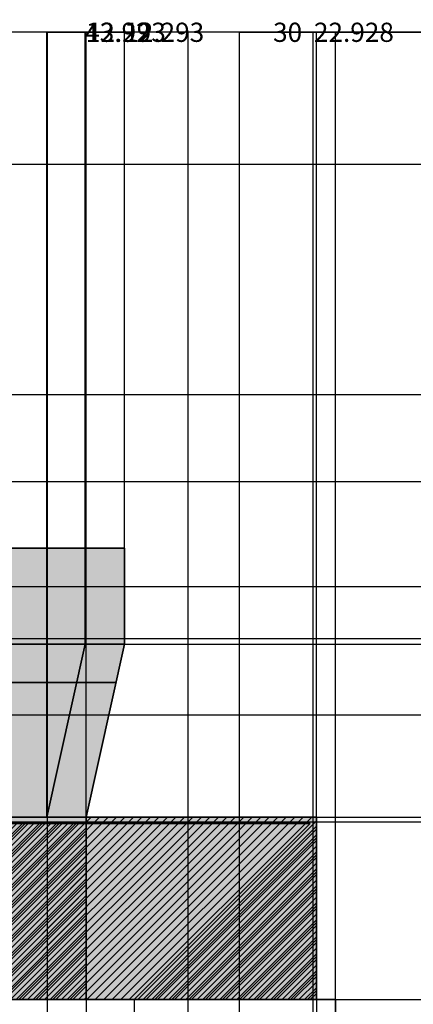
# Model space of a CAD drawing. Units: inches. Extents: x 148 to 1080, y 89 to 707.
# Tile 11 of 12: x 674 to 797, y 399 to 707. Entities that reach past the tile are written whole.
import ezdxf

# ---------------------------------------------------------------- set-up
doc = ezdxf.new("R2010")
doc.units = ezdxf.units.IN
doc.header["$MEASUREMENT"] = 0
for name, color, linetype, lineweight in [('A-ANNO-DIMS', 2, 'Continuous', 18), ('A-ELEV', 7, 'Continuous', 35), ('A-ELEV-PATT', 8, 'Continuous', 13)]:
    doc.layers.add(name, color=color, linetype=linetype, lineweight=lineweight)
doc.styles.get("Standard").update_dxf_attribs({"font": 'arial.ttf'})
doc.dimstyles.get("Standard").update_dxf_attribs({"dimtxt": 6, "dimasz": 0.18, "dimexe": 0.18, "dimexo": 0.0625, "dimgap": 0.09, "dimtad": 0, "dimtih": 1, "dimtoh": 1, "dimdec": 0, "dimzin": 0, "dimdsep": 46, "dimlunit": 3, "dimtxsty": 'Standard', "dimcen": 0.09, "dimadec": 0, "dimazin": 0, "dimtfac": 1, "dimtdec": 0, "dimtofl": 0, "dimtmove": 0, "dimatfit": 3, "dimfxl": 1, "dimtolj": 1, "dimtzin": 0, "dimarcsym": 0})

# ---------------------------------------------------------------- blocks, each defined once
blk = doc.blocks.new('*D1')
at = {"layer": 'A-ANNO-DIMS', "color": 0, "lineweight": -2, "transparency": 16777216}
for p, q in [((215.02, 662.01), (215.02, 703.28)), ((215.2, 703.1), (604.32, 703.1)), ((1006.77, 703.1), (617.65, 703.1)), ((1006.95, 338.01), (1006.95, 703.28))]:
    blk.add_line(p, q, dxfattribs=at)
at = {"layer": 'A-ANNO-DIMS', "color": 0, "transparency": 16777216}
for points in [[(215.2, 703.13), (215.2, 703.07), (215.02, 703.1)], [(1006.77, 703.13), (1006.77, 703.07), (1006.95, 703.1)]]:
    blk.add_solid(points, dxfattribs=at)
at = {"layer": 'Defpoints', "color": 0, "transparency": 16777216}
for p in [(1006.95, 703.1), (215.02, 661.95), (1006.95, 337.95)]:
    blk.add_point(p, dxfattribs=at)
at = {"layer": 'A-ANNO-DIMS', "color": 0, "transparency": 16777216, "insert": (610.98, 703.1), "char_height": 6, "attachment_point": 5}
blk.add_mtext('\\A1;792', dxfattribs=at)
blk = doc.blocks.new('*D14')
at = {"layer": 'A-ANNO-DIMS', "color": 0, "lineweight": -2, "transparency": 16777216}
for p, q in [((611.02, 542.01), (611.02, 703.28)), ((611.2, 703.1), (654.63, 703.1)), ((706.84, 703.1), (663.41, 703.1)), ((707.02, 542.01), (707.02, 703.28))]:
    blk.add_line(p, q, dxfattribs=at)
at = {"layer": 'A-ANNO-DIMS', "color": 0, "transparency": 16777216}
for points in [[(611.2, 703.13), (611.2, 703.07), (611.02, 703.1)], [(706.84, 703.13), (706.84, 703.07), (707.02, 703.1)]]:
    blk.add_solid(points, dxfattribs=at)
at = {"layer": 'Defpoints', "color": 0, "transparency": 16777216}
for p in [(707.02, 703.1), (611.02, 541.95), (707.02, 541.95)]:
    blk.add_point(p, dxfattribs=at)
at = {"layer": 'A-ANNO-DIMS', "color": 0, "transparency": 16777216, "insert": (659.02, 703.1), "char_height": 6, "attachment_point": 5}
blk.add_mtext('\\A1;96', dxfattribs=at)
blk = doc.blocks.new('*D16')
at = {"layer": 'A-ANNO-DIMS', "color": 0, "lineweight": -2, "transparency": 16777216}
for p, q in [((527.02, 458.01), (527.02, 703.28)), ((527.2, 703.1), (640.26, 703.1)), ((766.84, 703.1), (653.78, 703.1)), ((767.02, 458.01), (767.02, 703.28))]:
    blk.add_line(p, q, dxfattribs=at)
at = {"layer": 'A-ANNO-DIMS', "color": 0, "transparency": 16777216}
for points in [[(527.2, 703.13), (527.2, 703.07), (527.02, 703.1)], [(766.84, 703.13), (766.84, 703.07), (767.02, 703.1)]]:
    blk.add_solid(points, dxfattribs=at)
at = {"layer": 'Defpoints', "color": 0, "transparency": 16777216}
for p in [(767.02, 703.1), (527.02, 457.95), (767.02, 457.95)]:
    blk.add_point(p, dxfattribs=at)
at = {"layer": 'A-ANNO-DIMS', "color": 0, "transparency": 16777216, "insert": (647.02, 703.1), "char_height": 6, "attachment_point": 5}
blk.add_mtext('\\A1;240', dxfattribs=at)
blk = doc.blocks.new('*D17')
at = {"layer": 'A-ANNO-DIMS', "color": 0, "lineweight": -2, "transparency": 16777216}
for p, q in [((743.02, 338.01), (743.02, 703.28)), ((743.2, 703.1), (753.64, 703.1)), ((772.84, 703.1), (762.39, 703.1)), ((773.02, 368.01), (773.02, 703.28))]:
    blk.add_line(p, q, dxfattribs=at)
at = {"layer": 'A-ANNO-DIMS', "color": 0, "transparency": 16777216}
for points in [[(743.2, 703.13), (743.2, 703.07), (743.02, 703.1)], [(772.84, 703.13), (772.84, 703.07), (773.02, 703.1)]]:
    blk.add_solid(points, dxfattribs=at)
at = {"layer": 'Defpoints', "color": 0, "transparency": 16777216}
for p in [(773.02, 703.1), (773.02, 367.95), (743.02, 337.95)]:
    blk.add_point(p, dxfattribs=at)
at = {"layer": 'A-ANNO-DIMS', "color": 0, "transparency": 16777216, "insert": (758.02, 703.1), "char_height": 6, "attachment_point": 5}
blk.add_mtext('\\A1;30', dxfattribs=at)
blk = doc.blocks.new('*D18')
at = {"layer": 'A-ANNO-DIMS', "color": 0, "lineweight": -2, "transparency": 16777216}
for p, q in [((635.08, 661.95), (1064.5, 661.95)), ((1064.32, 661.77), (1064.32, 401.1)), ((1064.32, 134.13), (1064.32, 394.79)), ((1007.01, 133.95), (1064.5, 133.95))]:
    blk.add_line(p, q, dxfattribs=at)
at = {"layer": 'A-ANNO-DIMS', "color": 0, "transparency": 16777216}
for points in [[(1064.29, 661.77), (1064.35, 661.77), (1064.32, 661.95)], [(1064.29, 134.13), (1064.35, 134.13), (1064.32, 133.95)]]:
    blk.add_solid(points, dxfattribs=at)
at = {"layer": 'Defpoints', "color": 0, "transparency": 16777216}
for p in [(635.02, 661.95), (1064.32, 661.95), (1006.95, 133.95)]:
    blk.add_point(p, dxfattribs=at)
at = {"layer": 'A-ANNO-DIMS', "color": 0, "transparency": 16777216, "insert": (1064.32, 397.95), "char_height": 6, "attachment_point": 5}
blk.add_mtext('\\A1;528', dxfattribs=at)
blk = doc.blocks.new('*D35')
at = {"layer": 'A-ANNO-DIMS', "color": 0, "lineweight": -2, "transparency": 16777216}
for p, q in [((743.02, 272.01), (743.02, 703.28)), ((743.2, 703.1), (765.77, 703.1)), ((765.95, 241.16), (765.95, 703.28)), ((765.95, 703.1), (766.13, 703.1))]:
    blk.add_line(p, q, dxfattribs=at)
at = {"layer": 'A-ANNO-DIMS', "color": 0, "transparency": 16777216}
for points in [[(743.2, 703.13), (743.2, 703.07), (743.02, 703.1)], [(765.77, 703.13), (765.77, 703.07), (765.95, 703.1)]]:
    blk.add_solid(points, dxfattribs=at)
at = {"layer": 'Defpoints', "color": 0, "transparency": 16777216}
for p in [(765.95, 703.1), (743.02, 271.95), (765.95, 241.1)]:
    blk.add_point(p, dxfattribs=at)
at = {"layer": 'A-ANNO-DIMS', "color": 0, "transparency": 16777216, "insert": (778.73, 703.1), "char_height": 6, "attachment_point": 5}
blk.add_mtext('\\A1;22.928', dxfattribs=at)
blk = doc.blocks.new('*D36')
at = {"layer": 'A-ANNO-DIMS', "color": 0, "lineweight": -2, "transparency": 16777216}
for p, q in [((765.95, 241.16), (765.95, 703.28)), ((766.13, 703.1), (844.01, 703.1)), ((934.77, 703.1), (856.89, 703.1)), ((934.95, 272.01), (934.95, 703.28))]:
    blk.add_line(p, q, dxfattribs=at)
at = {"layer": 'A-ANNO-DIMS', "color": 0, "transparency": 16777216}
for points in [[(766.13, 703.13), (766.13, 703.07), (765.95, 703.1)], [(934.77, 703.13), (934.77, 703.07), (934.95, 703.1)]]:
    blk.add_solid(points, dxfattribs=at)
at = {"layer": 'Defpoints', "color": 0, "transparency": 16777216}
for p in [(934.95, 703.1), (934.95, 271.95), (765.95, 241.1)]:
    blk.add_point(p, dxfattribs=at)
at = {"layer": 'A-ANNO-DIMS', "color": 0, "transparency": 16777216, "insert": (850.45, 703.1), "char_height": 6, "attachment_point": 5}
blk.add_mtext('\\A1;169', dxfattribs=at)
blk = doc.blocks.new('*D37')
at = {"layer": 'A-ANNO-DIMS', "color": 0, "lineweight": -2, "transparency": 16777216}
for p, q in [((765.95, 241.16), (765.95, 703.28)), ((766.13, 703.1), (836.75, 703.1)), ((927.28, 703.1), (856.66, 703.1)), ((927.46, 240.26), (927.46, 703.28))]:
    blk.add_line(p, q, dxfattribs=at)
at = {"layer": 'A-ANNO-DIMS', "color": 0, "transparency": 16777216}
for points in [[(766.13, 703.13), (766.13, 703.07), (765.95, 703.1)], [(927.28, 703.13), (927.28, 703.07), (927.46, 703.1)]]:
    blk.add_solid(points, dxfattribs=at)
at = {"layer": 'Defpoints', "color": 0, "transparency": 16777216}
for p in [(927.46, 703.1), (765.95, 241.1), (927.46, 240.2)]:
    blk.add_point(p, dxfattribs=at)
at = {"layer": 'A-ANNO-DIMS', "color": 0, "transparency": 16777216, "insert": (846.7, 703.1), "char_height": 6, "attachment_point": 5}
blk.add_mtext('\\A1;161.5', dxfattribs=at)
blk = doc.blocks.new('*D47')
at = {"layer": 'A-ANNO-DIMS', "color": 0, "lineweight": -2, "transparency": 16777216}
for p, q in [((628.17, 353.26), (628.17, 703.28)), ((628.35, 703.1), (645.36, 703.1)), ((682.84, 703.1), (665.83, 703.1)), ((683.02, 338.01), (683.02, 703.28))]:
    blk.add_line(p, q, dxfattribs=at)
at = {"layer": 'A-ANNO-DIMS', "color": 0, "transparency": 16777216}
for points in [[(628.35, 703.13), (628.35, 703.07), (628.17, 703.1)], [(682.84, 703.13), (682.84, 703.07), (683.02, 703.1)]]:
    blk.add_solid(points, dxfattribs=at)
at = {"layer": 'Defpoints', "color": 0, "transparency": 16777216}
for p in [(683.02, 703.1), (628.17, 353.2), (683.02, 337.95)]:
    blk.add_point(p, dxfattribs=at)
at = {"layer": 'A-ANNO-DIMS', "color": 0, "transparency": 16777216, "insert": (655.6, 703.1), "char_height": 6, "attachment_point": 5}
blk.add_mtext('\\A1;54.85', dxfattribs=at)
blk = doc.blocks.new('*D48')
at = {"layer": 'A-ANNO-DIMS', "color": 0, "lineweight": -2, "transparency": 16777216}
for p, q in [((683.02, 338.01), (683.02, 703.28)), ((683.2, 703.1), (694.68, 703.1)), ((726.76, 703.1), (715.28, 703.1)), ((726.94, 354.92), (726.94, 703.28))]:
    blk.add_line(p, q, dxfattribs=at)
at = {"layer": 'A-ANNO-DIMS', "color": 0, "transparency": 16777216}
for points in [[(683.2, 703.13), (683.2, 703.07), (683.02, 703.1)], [(726.76, 703.13), (726.76, 703.07), (726.94, 703.1)]]:
    blk.add_solid(points, dxfattribs=at)
at = {"layer": 'Defpoints', "color": 0, "transparency": 16777216}
for p in [(726.94, 703.1), (726.94, 354.86), (683.02, 337.95)]:
    blk.add_point(p, dxfattribs=at)
at = {"layer": 'A-ANNO-DIMS', "color": 0, "transparency": 16777216, "insert": (704.98, 703.1), "char_height": 6, "attachment_point": 5}
blk.add_mtext('\\A1;43.92', dxfattribs=at)
blk = doc.blocks.new('*D51')
at = {"layer": 'A-ANNO-DIMS', "color": 0, "lineweight": -2, "transparency": 16777216}
for p, q in [((707.08, 511.95), (1064.5, 511.95)), ((1064.32, 511.77), (1064.32, 488.1)), ((1064.32, 458.13), (1064.32, 481.79)), ((695.08, 457.95), (1064.5, 457.95))]:
    blk.add_line(p, q, dxfattribs=at)
at = {"layer": 'A-ANNO-DIMS', "color": 0, "transparency": 16777216}
for points in [[(1064.29, 511.77), (1064.35, 511.77), (1064.32, 511.95)], [(1064.29, 458.13), (1064.35, 458.13), (1064.32, 457.95)]]:
    blk.add_solid(points, dxfattribs=at)
at = {"layer": 'Defpoints', "color": 0, "transparency": 16777216}
for p in [(707.02, 511.95), (695.02, 457.95), (1064.32, 457.95)]:
    blk.add_point(p, dxfattribs=at)
at = {"layer": 'A-ANNO-DIMS', "color": 0, "transparency": 16777216, "insert": (1064.32, 484.95), "char_height": 6, "attachment_point": 5}
blk.add_mtext('\\A1;54.00', dxfattribs=at)
blk = doc.blocks.new('*D53')
at = {"layer": 'A-ANNO-DIMS', "color": 0, "lineweight": -2, "transparency": 16777216}
for p, q in [((694.73, 512.01), (694.73, 703.28)), ((694.91, 703.1), (706.84, 703.1)), ((707.02, 512.01), (707.02, 703.28)), ((707.02, 703.1), (707.2, 703.1))]:
    blk.add_line(p, q, dxfattribs=at)
at = {"layer": 'A-ANNO-DIMS', "color": 0, "transparency": 16777216}
for points in [[(694.91, 703.13), (694.91, 703.07), (694.73, 703.1)], [(706.84, 703.13), (706.84, 703.07), (707.02, 703.1)]]:
    blk.add_solid(points, dxfattribs=at)
at = {"layer": 'Defpoints', "color": 0, "transparency": 16777216}
for p in [(707.02, 703.1), (694.73, 511.95), (707.02, 511.95)]:
    blk.add_point(p, dxfattribs=at)
at = {"layer": 'A-ANNO-DIMS', "color": 0, "transparency": 16777216, "insert": (719.46, 703.1), "char_height": 6, "attachment_point": 5}
blk.add_mtext('\\A1;12.293', dxfattribs=at)
blk = doc.blocks.new('*D54')
at = {"layer": 'A-ANNO-DIMS', "color": 0, "lineweight": -2, "transparency": 16777216}
for p, q in [((682.73, 458.01), (682.73, 703.28)), ((682.91, 703.1), (694.84, 703.1)), ((695.02, 458.01), (695.02, 703.28)), ((695.02, 703.1), (695.2, 703.1))]:
    blk.add_line(p, q, dxfattribs=at)
at = {"layer": 'A-ANNO-DIMS', "color": 0, "transparency": 16777216}
for points in [[(682.91, 703.13), (682.91, 703.07), (682.73, 703.1)], [(694.84, 703.13), (694.84, 703.07), (695.02, 703.1)]]:
    blk.add_solid(points, dxfattribs=at)
at = {"layer": 'Defpoints', "color": 0, "transparency": 16777216}
for p in [(695.02, 703.1), (682.73, 457.95), (695.02, 457.95)]:
    blk.add_point(p, dxfattribs=at)
at = {"layer": 'A-ANNO-DIMS', "color": 0, "transparency": 16777216, "insert": (707.46, 703.1), "char_height": 6, "attachment_point": 5}
blk.add_mtext('\\A1;12.293', dxfattribs=at)
blk = doc.blocks.new('*D58')
at = {"layer": 'A-ANNO-DIMS', "color": 0, "lineweight": -2, "transparency": 16777216}
for p, q in [((611.02, 400.88), (611.02, 92.62)), ((695.02, 400.88), (695.02, 92.62)), ((611.2, 92.8), (642.81, 92.8)), ((694.84, 92.8), (663.23, 92.8))]:
    blk.add_line(p, q, dxfattribs=at)
at = {"layer": 'A-ANNO-DIMS', "color": 0, "transparency": 16777216}
for points in [[(611.2, 92.83), (611.2, 92.77), (611.02, 92.8)], [(694.84, 92.83), (694.84, 92.77), (695.02, 92.8)]]:
    blk.add_solid(points, dxfattribs=at)
at = {"layer": 'Defpoints', "color": 0, "transparency": 16777216}
for p in [(611.02, 400.95), (695.02, 400.95), (695.02, 92.8)]:
    blk.add_point(p, dxfattribs=at)
at = {"layer": 'A-ANNO-DIMS', "color": 0, "transparency": 16777216, "insert": (653.02, 92.8), "char_height": 6, "attachment_point": 5}
blk.add_mtext('\\A1;84.00', dxfattribs=at)
blk = doc.blocks.new('*D59')
at = {"layer": 'A-ANNO-DIMS', "color": 0, "lineweight": -2, "transparency": 16777216}
for p, q in [((695.02, 400.88), (695.02, 92.62)), ((767.02, 400.88), (767.02, 92.62)), ((695.2, 92.8), (720.84, 92.8)), ((766.84, 92.8), (741.2, 92.8))]:
    blk.add_line(p, q, dxfattribs=at)
at = {"layer": 'A-ANNO-DIMS', "color": 0, "transparency": 16777216}
for points in [[(695.2, 92.83), (695.2, 92.77), (695.02, 92.8)], [(766.84, 92.83), (766.84, 92.77), (767.02, 92.8)]]:
    blk.add_solid(points, dxfattribs=at)
at = {"layer": 'Defpoints', "color": 0, "transparency": 16777216}
for p in [(695.02, 400.95), (767.02, 400.95), (767.02, 92.8)]:
    blk.add_point(p, dxfattribs=at)
at = {"layer": 'A-ANNO-DIMS', "color": 0, "transparency": 16777216, "insert": (731.02, 92.8), "char_height": 6, "attachment_point": 5}
blk.add_mtext('\\A1;72.00', dxfattribs=at)
blk = doc.blocks.new('*D60')
at = {"layer": 'A-ANNO-DIMS', "color": 0, "lineweight": -2, "transparency": 16777216}
for p, q in [((695.02, 400.88), (695.02, 92.62)), ((710.1, 400.88), (710.1, 92.62)), ((695.2, 92.8), (709.92, 92.8)), ((710.1, 92.8), (710.28, 92.8))]:
    blk.add_line(p, q, dxfattribs=at)
at = {"layer": 'A-ANNO-DIMS', "color": 0, "transparency": 16777216}
for points in [[(695.2, 92.83), (695.2, 92.77), (695.02, 92.8)], [(709.92, 92.83), (709.92, 92.77), (710.1, 92.8)]]:
    blk.add_solid(points, dxfattribs=at)
at = {"layer": 'Defpoints', "color": 0, "transparency": 16777216}
for p in [(695.02, 400.95), (710.1, 400.95), (710.1, 92.8)]:
    blk.add_point(p, dxfattribs=at)
at = {"layer": 'A-ANNO-DIMS', "color": 0, "transparency": 16777216, "insert": (720.22, 92.8), "char_height": 6, "attachment_point": 5}
blk.add_mtext('\\A1;15.08', dxfattribs=at)
blk = doc.blocks.new('*D90')
at = {"layer": 'A-ANNO-DIMS', "color": 0, "lineweight": -2, "transparency": 16777216}
for p, q in [((527.08, 489.89), (1064.5, 489.89)), ((1064.32, 489.71), (1064.32, 448.57)), ((1064.32, 401.13), (1064.32, 442.27)), ((527.08, 400.95), (1064.5, 400.95))]:
    blk.add_line(p, q, dxfattribs=at)
at = {"layer": 'A-ANNO-DIMS', "color": 0, "transparency": 16777216}
for points in [[(1064.29, 489.71), (1064.35, 489.71), (1064.32, 489.89)], [(1064.29, 401.13), (1064.35, 401.13), (1064.32, 400.95)]]:
    blk.add_solid(points, dxfattribs=at)
at = {"layer": 'Defpoints', "color": 0, "transparency": 16777216}
for p in [(527.02, 489.89), (527.02, 400.95), (1064.32, 400.95)]:
    blk.add_point(p, dxfattribs=at)
at = {"layer": 'A-ANNO-DIMS', "color": 0, "transparency": 16777216, "insert": (1064.32, 445.42), "char_height": 6, "attachment_point": 5}
blk.add_mtext('\\A1;88.94', dxfattribs=at)
blk = doc.blocks.new('*D91')
at = {"layer": 'A-ANNO-DIMS', "color": 0, "lineweight": -2, "transparency": 16777216}
for p, q in [((479.08, 513.77), (1064.5, 513.77)), ((1064.32, 513.59), (1064.32, 460.51)), ((1064.32, 401.13), (1064.32, 454.21)), ((479.08, 400.95), (1064.5, 400.95))]:
    blk.add_line(p, q, dxfattribs=at)
at = {"layer": 'A-ANNO-DIMS', "color": 0, "transparency": 16777216}
for points in [[(1064.29, 513.59), (1064.35, 513.59), (1064.32, 513.77)], [(1064.29, 401.13), (1064.35, 401.13), (1064.32, 400.95)]]:
    blk.add_solid(points, dxfattribs=at)
at = {"layer": 'Defpoints', "color": 0, "transparency": 16777216}
for p in [(479.02, 513.77), (479.02, 400.95), (1064.32, 400.95)]:
    blk.add_point(p, dxfattribs=at)
at = {"layer": 'A-ANNO-DIMS', "color": 0, "transparency": 16777216, "insert": (1064.32, 457.36), "char_height": 6, "attachment_point": 5}
blk.add_mtext('\\A1;112.82', dxfattribs=at)
blk = doc.blocks.new('*D92')
at = {"layer": 'A-ANNO-DIMS', "color": 0, "lineweight": -2, "transparency": 16777216}
for p, q in [((389.08, 456.43), (1064.5, 456.43)), ((1064.32, 456.25), (1064.32, 431.84)), ((1064.32, 401.13), (1064.32, 425.53)), ((389.08, 400.95), (1064.5, 400.95))]:
    blk.add_line(p, q, dxfattribs=at)
at = {"layer": 'A-ANNO-DIMS', "color": 0, "transparency": 16777216}
for points in [[(1064.29, 456.25), (1064.35, 456.25), (1064.32, 456.43)], [(1064.29, 401.13), (1064.35, 401.13), (1064.32, 400.95)]]:
    blk.add_solid(points, dxfattribs=at)
at = {"layer": 'Defpoints', "color": 0, "transparency": 16777216}
for p in [(389.02, 456.43), (1064.32, 456.43), (389.02, 400.95)]:
    blk.add_point(p, dxfattribs=at)
at = {"layer": 'A-ANNO-DIMS', "color": 0, "transparency": 16777216, "insert": (1064.32, 428.69), "char_height": 6, "attachment_point": 5}
blk.add_mtext('\\A1;55.48', dxfattribs=at)
blk = doc.blocks.new('*D93')
at = {"layer": 'A-ANNO-DIMS', "color": 0, "lineweight": -2, "transparency": 16777216}
for p, q in [((389.08, 529.95), (1064.5, 529.95)), ((1064.32, 529.77), (1064.32, 496.34)), ((1064.32, 456.61), (1064.32, 490.03)), ((389.08, 456.43), (1064.5, 456.43))]:
    blk.add_line(p, q, dxfattribs=at)
at = {"layer": 'A-ANNO-DIMS', "color": 0, "transparency": 16777216}
for points in [[(1064.29, 529.77), (1064.35, 529.77), (1064.32, 529.95)], [(1064.29, 456.61), (1064.35, 456.61), (1064.32, 456.43)]]:
    blk.add_solid(points, dxfattribs=at)
at = {"layer": 'Defpoints', "color": 0, "transparency": 16777216}
for p in [(389.02, 529.95), (1064.32, 529.95), (389.02, 456.43)]:
    blk.add_point(p, dxfattribs=at)
at = {"layer": 'A-ANNO-DIMS', "color": 0, "transparency": 16777216, "insert": (1064.32, 493.19), "char_height": 6, "attachment_point": 5}
blk.add_mtext('\\A1;73.52', dxfattribs=at)
blk = doc.blocks.new('*D94')
at = {"layer": 'A-ANNO-DIMS', "color": 0, "lineweight": -2, "transparency": 16777216}
for p, q in [((389.08, 562.74), (1064.5, 562.74)), ((1064.32, 562.56), (1064.32, 549.5)), ((1064.32, 530.13), (1064.32, 543.19)), ((389.08, 529.95), (1064.5, 529.95))]:
    blk.add_line(p, q, dxfattribs=at)
at = {"layer": 'A-ANNO-DIMS', "color": 0, "transparency": 16777216}
for points in [[(1064.29, 562.56), (1064.35, 562.56), (1064.32, 562.74)], [(1064.29, 530.13), (1064.35, 530.13), (1064.32, 529.95)]]:
    blk.add_solid(points, dxfattribs=at)
at = {"layer": 'Defpoints', "color": 0, "transparency": 16777216}
for p in [(389.02, 562.74), (1064.32, 562.74), (389.02, 529.95)]:
    blk.add_point(p, dxfattribs=at)
at = {"layer": 'A-ANNO-DIMS', "color": 0, "transparency": 16777216, "insert": (1064.32, 546.34), "char_height": 6, "attachment_point": 5}
blk.add_mtext('\\A1;32.79', dxfattribs=at)
blk = doc.blocks.new('*D95')
at = {"layer": 'A-ANNO-DIMS', "color": 0, "lineweight": -2, "transparency": 16777216}
for p, q in [((389.08, 589.95), (1064.5, 589.95)), ((1064.32, 589.77), (1064.32, 579.44)), ((1064.32, 562.92), (1064.32, 573.24)), ((389.08, 562.74), (1064.5, 562.74))]:
    blk.add_line(p, q, dxfattribs=at)
at = {"layer": 'A-ANNO-DIMS', "color": 0, "transparency": 16777216}
for points in [[(1064.29, 589.77), (1064.35, 589.77), (1064.32, 589.95)], [(1064.29, 562.92), (1064.35, 562.92), (1064.32, 562.74)]]:
    blk.add_solid(points, dxfattribs=at)
at = {"layer": 'Defpoints', "color": 0, "transparency": 16777216}
for p in [(389.02, 589.95), (1064.32, 589.95), (389.02, 562.74)]:
    blk.add_point(p, dxfattribs=at)
at = {"layer": 'A-ANNO-DIMS', "color": 0, "transparency": 16777216, "insert": (1064.32, 576.34), "char_height": 6, "attachment_point": 5}
blk.add_mtext('\\A1;27.21', dxfattribs=at)

msp = doc.modelspace()

# ---------------------------------------------------------------- hatches: boundary and pattern name
at = {"layer": 'A-ELEV-PATT'}
h = msp.add_hatch(color=256, dxfattribs=at)
h.dxf.hatch_style = 1
h.paths.add_polyline_path([(707.0199, 511.9474), (707.0199, 541.9474), (611.0199, 541.9474), (611.0199, 511.9474)])
h.paths.add_polyline_path([(479.0199, 513.7706), (395.0199, 513.7706), (395.0199, 400.9474), (479.0199, 400.9474)])
h = msp.add_hatch(color=256, dxfattribs=at)
h.dxf.hatch_style = 1
h.paths.add_polyline_path([(694.7271, 511.9474), (611.0199, 511.9474), (611.0199, 499.9474), (692.0605, 499.9474)])
h.paths.add_polyline_path([(692.0605, 499.9474), (611.0199, 499.9474), (611.0199, 457.9474), (682.7271, 457.9474)])
h.paths.add_polyline_path([(704.3532, 499.9474), (692.0605, 499.9474), (682.7271, 457.9474), (695.0199, 457.9474)])
h.paths.add_polyline_path([(707.0199, 511.9474), (694.7271, 511.9474), (692.0605, 499.9474), (704.3532, 499.9474)])
h = msp.add_hatch(color=256, dxfattribs=at)
h.dxf.hatch_style = 1
h.paths.add_polyline_path([(695.0199, 457.9474), (611.0199, 457.9474), (611.0199, 455.9474), (695.0199, 455.9474)])
h.paths.add_polyline_path([(611.0199, 457.9474), (527.0199, 457.9474), (527.0199, 455.9474), (611.0199, 455.9474)])
h = msp.add_hatch(dxfattribs=at)
h.set_pattern_fill('ANSI31', color=256, scale=15)
h.paths.add_polyline_path([(611.0199, 455.9474), (527.0199, 455.9474), (527.0199, 400.9474), (611.0199, 400.9474)])
h.paths.add_polyline_path([(695.0199, 455.9474), (611.0199, 455.9474), (611.0199, 400.9474), (695.0199, 400.9474)])
h.paths.add_polyline_path([(765.0227, 455.9474), (695.0199, 455.9474), (695.0199, 400.9474), (710.0996, 400.9474)], flags=17)
h.paths.add_polyline_path([(767.0199, 455.117), (767.0199, 457.9474), (695.0199, 457.9474), (695.0199, 455.9474), (765.0227, 455.9474), (710.0996, 400.9474), (712.9261, 400.9474)])
h.paths.add_polyline_path([(767.0199, 455.117), (712.9261, 400.9474), (767.0199, 400.9474)])
h = msp.add_hatch(color=256, dxfattribs=at)
h.dxf.hatch_style = 1
h.paths.add_polyline_path([(611.0199, 455.9474), (527.0199, 455.9474), (527.0199, 400.9474), (611.0199, 400.9474)])
h.paths.add_polyline_path([(765.0227, 455.9474), (695.0199, 455.9474), (695.0199, 400.9474), (710.0996, 400.9474)])
h = msp.add_hatch(color=256, dxfattribs=at)
h.dxf.hatch_style = 1
h.paths.add_polyline_path([(695.0199, 455.9474), (611.0199, 455.9474), (611.0199, 400.9474), (695.0199, 400.9474)])
h.paths.add_polyline_path([(767.0199, 455.117), (712.9261, 400.9474), (767.0199, 400.9474)])
h = msp.add_hatch(dxfattribs=at)
h.set_pattern_fill('ANSI31', color=256, scale=10)
h.paths.add_polyline_path([(767.0199, 455.117), (712.9261, 400.9474), (767.0199, 400.9474)])
h.paths.add_polyline_path([(695.0199, 455.9474), (611.0199, 455.9474), (611.0199, 400.9474), (695.0199, 400.9474)])
h = msp.add_hatch(color=256, dxfattribs=at)
h.dxf.hatch_style = 1
h.paths.add_polyline_path([(767.0199, 457.9474), (695.0199, 457.9474), (695.0199, 455.9474), (765.0227, 455.9474), (710.0996, 400.9474), (712.9261, 400.9474), (767.0199, 455.117)])

# ---------------------------------------------------------------- linework, layer by layer
at = {"layer": 'A-ELEV'}
for p, q in [((527.0199, 541.9474), (707.0199, 541.9474)), ((707.0199, 511.9474), (707.0199, 541.9474)), ((611.0199, 511.9474), (707.0199, 511.9474)), ((694.7271, 511.9474), (682.7271, 457.9474)), ((707.0199, 511.9474), (695.0199, 457.9474)), ((611.0199, 499.9474), (704.3532, 499.9474)), ((527.0199, 457.9474), (767.0199, 457.9474)), ((527.0199, 455.9474), (765.0227, 455.9474)), ((695.0199, 400.9474), (695.0199, 457.9474)), ((765.0227, 455.9474), (710.0996, 400.9474)), ((767.0199, 400.9474), (767.0199, 457.9474)), ((767.0199, 455.117), (712.9261, 400.9474)), ((215.0199, 400.9474), (773.0199, 400.9474)), ((773.0199, 367.9474), (773.0199, 400.9474))]:
    msp.add_line(p, q, dxfattribs=at)

# ---------------------------------------------------------------- dimensions: what is measured, and where the dimension line sits
at = {"layer": 'A-ANNO-DIMS'}
for base, p1, p2, override, picture, middle in [((1006.9492, 703.0974), (215.0199, 661.9474), (1006.9492, 337.9474), {"dimdec": 0, "dimlfac": 1, "dimrnd": 0, "dimzin": 0, "dimdsep": 46, "dimlunit": 2}, '*D1', (610.9845, 703.0974)), ((767.0199, 703.0974), (527.0199, 457.9474), (767.0199, 457.9474), {"dimdec": 0, "dimlfac": 1, "dimrnd": 0, "dimzin": 0, "dimdsep": 46, "dimlunit": 2}, '*D16', (647.0199, 703.0974)), ((707.0199, 703.0974), (611.0199, 541.9474), (707.0199, 541.9474), {"dimdec": 0, "dimlfac": 1, "dimrnd": 0, "dimzin": 0, "dimdsep": 46, "dimlunit": 2}, '*D14', (659.0199, 703.0974)), ((683.0199, 703.0974), (628.1736, 353.1958), (683.0199, 337.9474), {"dimdec": 2, "dimlfac": 1, "dimrnd": 0, "dimzin": 0, "dimdsep": 46, "dimlunit": 2}, '*D47', (655.5968, 703.0974)), ((695.0199, 703.0974), (682.7271, 457.9474), (695.0199, 457.9474), {"dimdec": 3, "dimlfac": 1, "dimrnd": 0, "dimzin": 0, "dimdsep": 46, "dimlunit": 2}, '*D54', (707.4618, 703.0974)), ((726.9419, 703.0974), (683.0199, 337.9474), (726.9419, 354.8591), {"dimdec": 2, "dimlfac": 1, "dimrnd": 0, "dimzin": 0, "dimdsep": 46, "dimlunit": 2}, '*D48', (704.9809, 703.0974)), ((707.0199, 703.0974), (694.7271, 511.9474), (707.0199, 511.9474), {"dimdec": 3, "dimlfac": 1, "dimrnd": 0, "dimzin": 0, "dimdsep": 46, "dimlunit": 2}, '*D53', (719.4618, 703.0974)), ((773.0199, 703.0974), (743.0199, 337.9474), (773.0199, 367.9474), {"dimdec": 0, "dimlfac": 1, "dimrnd": 0, "dimzin": 0, "dimdsep": 46, "dimlunit": 2}, '*D17', (758.0199, 703.0974)), ((765.947371, 703.097395), (743.019868, 271.947395), (765.947371, 241.09963), {"dimdec": 3, "dimlfac": 1, "dimrnd": 0, "dimzin": 0, "dimdsep": 46, "dimlunit": 2}, '*D35', (778.728967, 703.097395)), ((934.9492, 703.0974), (765.9474, 241.0996), (934.9492, 271.9474), {"dimdec": 0, "dimlfac": 1, "dimrnd": 0, "dimzin": 0, "dimdsep": 46, "dimlunit": 2}, '*D36', (850.4483, 703.0974)), ((927.4587, 703.0974), (765.9474, 241.0996), (927.4587, 240.1966), {"dimdec": 1, "dimlfac": 1, "dimrnd": 0, "dimzin": 0, "dimdsep": 46, "dimlunit": 2}, '*D37', (846.703, 703.0974)), ((695.0199, 92.7974), (611.0199, 400.9474), (695.0199, 400.9474), {"dimdec": 2, "dimlfac": 1, "dimrnd": 0, "dimzin": 0, "dimdsep": 46, "dimlunit": 2}, '*D58', (653.0199, 92.7974)), ((767.0199, 92.7974), (695.0199, 400.9474), (767.0199, 400.9474), {"dimdec": 2, "dimlfac": 1, "dimrnd": 0, "dimzin": 0, "dimdsep": 46, "dimlunit": 2}, '*D59', (731.0199, 92.7974)), ((710.0996, 92.7974), (695.0199, 400.9474), (710.0996, 400.9474), {"dimdec": 2, "dimlfac": 1, "dimrnd": 0, "dimzin": 0, "dimdsep": 46, "dimlunit": 2}, '*D60', (720.2168, 92.7974))]:
    dim = msp.add_linear_dim(base=base, p1=p1, p2=p2, dimstyle='Standard', override=override, dxfattribs=at)
    dim.commit()
    dim.dimension.update_dxf_attribs({"geometry": picture, "text_midpoint": middle})
for base, p1, p2, override, picture, middle in [((1064.325, 661.9474), (1006.9492, 133.9474), (635.0199, 661.9474), {"dimdec": 0, "dimlfac": 1, "dimrnd": 0, "dimzin": 0, "dimdsep": 46, "dimlunit": 2}, '*D18', (1064.325, 397.9474)), ((1064.325, 589.9474), (389.0199, 562.736), (389.0199, 589.9474), {"dimdec": 2, "dimlfac": 1, "dimrnd": 0, "dimzin": 0, "dimdsep": 46, "dimlunit": 2}, '*D95', (1064.325, 576.3417)), ((1064.325, 562.736), (389.0199, 529.9474), (389.0199, 562.736), {"dimdec": 2, "dimlfac": 1, "dimrnd": 0, "dimzin": 0, "dimdsep": 46, "dimlunit": 2}, '*D94', (1064.325, 546.3417)), ((1064.325, 529.9474), (389.0199, 456.4274), (389.0199, 529.9474), {"dimdec": 2, "dimlfac": 1, "dimrnd": 0, "dimzin": 0, "dimdsep": 46, "dimlunit": 2}, '*D93', (1064.325, 493.1874)), ((1064.325, 400.9474), (479.0199, 513.7706), (479.0199, 400.9474), {"dimdec": 2, "dimlfac": 1, "dimrnd": 0, "dimzin": 0, "dimdsep": 46, "dimlunit": 2}, '*D91', (1064.325, 457.359)), ((1064.325, 457.9474), (707.0199, 511.9474), (695.0199, 457.9474), {"dimdec": 2, "dimlfac": 1, "dimrnd": 0, "dimzin": 0, "dimdsep": 46, "dimlunit": 2}, '*D51', (1064.325, 484.9474)), ((1064.325, 400.9474), (527.0199, 489.89), (527.0199, 400.9474), {"dimdec": 2, "dimlfac": 1, "dimrnd": 0, "dimzin": 0, "dimdsep": 46, "dimlunit": 2}, '*D90', (1064.325, 445.4187)), ((1064.325, 456.4274), (389.0199, 400.9474), (389.0199, 456.4274), {"dimdec": 2, "dimlfac": 1, "dimrnd": 0, "dimzin": 0, "dimdsep": 46, "dimlunit": 2}, '*D92', (1064.325, 428.6874))]:
    dim = msp.add_linear_dim(base=base, p1=p1, p2=p2, angle=90, dimstyle='Standard', override=override, dxfattribs=at)
    dim.commit()
    dim.dimension.update_dxf_attribs({"geometry": picture, "text_midpoint": middle})

doc.saveas('drawing.dxf')
